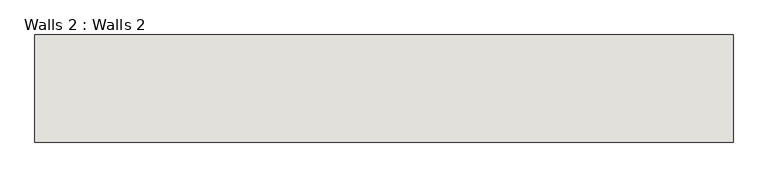
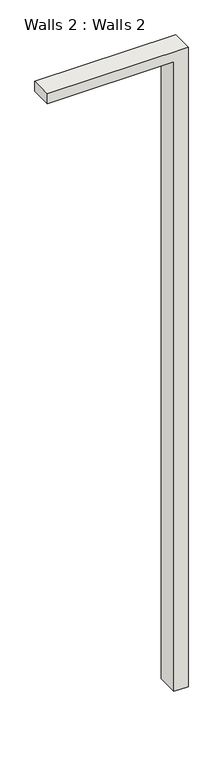
"""IFC4 building model written with IfcOpenShell, lengths in millimetres: wall geometry, Walls 2 : Walls 2."""

from ifc_helpers import new_model, si_unit, frame, origin, place, context, project, spatial, polyline, outline, extrude, source, transform, mapped, element, save


def walls_2_walls_2_973aa2a3(model_context):
    return source(origin(), model_context, "Body", "SweptSolid", [
        extrude(outline(polyline([(9118.6695108, -4193.9407032), (9118.6695108, -6175.1407032), (8970.5998721, -6175.1407032), (8970.5998721, -4393.9407032), (-400.0, -4393.9407032), (-400.0, -4193.9407032), (9118.6695108, -4193.9407032)])), frame((0.0, 3251.3956099, 0.0), z_axis=(0.0, 1.0, 0.0), x_axis=(0.0, 0.0, 1.0)), (0.0, 0.0, 1.0), 304.8),
    ])


if __name__ == "__main__":
    model = new_model("IFC4")
    model_context = context("Model", 3, world=origin())
    ifc_project = project(units=[si_unit("LENGTHUNIT", "METRE", prefix="MILLI")], contexts=[model_context])
    site = spatial("IfcSite", under=ifc_project)
    building = spatial("IfcBuilding", under=site)
    placement = place(None, origin())
    walls_2_walls_2_shape = walls_2_walls_2_973aa2a3(model_context)
    element("IfcWall", 1, ObjectType="Walls 2 : Walls 2", at=placement, inside=building, context=model_context, shape_type="MappedRepresentation", body=[
        mapped(walls_2_walls_2_shape, transform((0.0, 0.0, 0.0), x_axis=(1.0, 0.0, 0.0), y_axis=(0.0, 1.0, 0.0), z_axis=(0.0, 0.0, 1.0))),
    ])
    save(model, "model.ifc")

# Revit data of these elements
# Element 1 (IfcWall, "Walls 2 : Walls 2")
#   Materials on its faces: "Default Wall"
# Materials
#   "Default Wall": colour RGB 80 80 80, transparency 0
